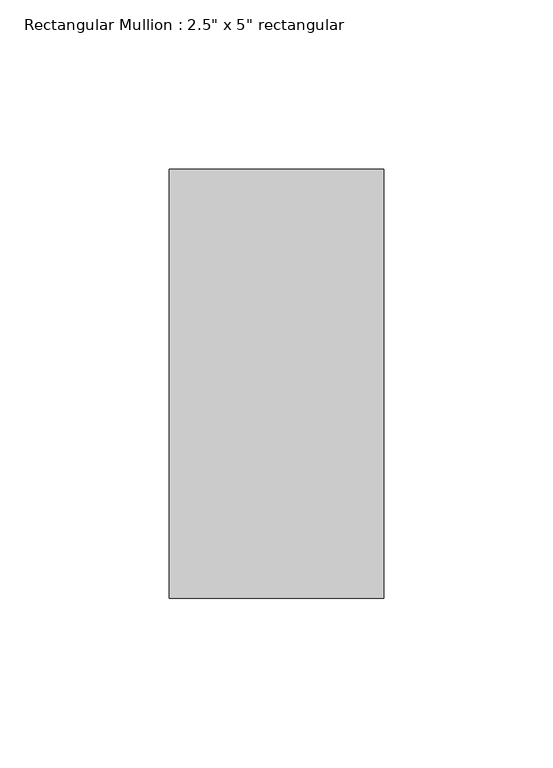
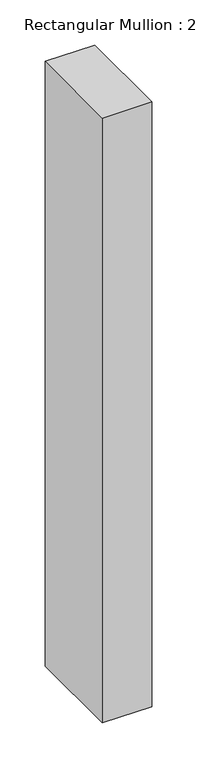
"""IFC4 building model written with IfcOpenShell, lengths in millimetres: member geometry."""

from ifc_helpers import new_model, si_unit, frame, origin, place, context, project, spatial, polyline, outline, extrude, source, transform, mapped, element, save


def member_ad567e07(model_context):
    return source(origin(), model_context, "Body", "SweptSolid", [
        extrude(outline(polyline([(31.75, 63.5), (31.75, -63.5), (-31.75, -63.5), (-31.75, 63.5), (31.75, 63.5)])), frame((0.0, 0.0, -819.15), z_axis=(0.0, 0.0, 1.0), x_axis=(1.0, 0.0, 0.0)), (0.0, 0.0, 1.0), 819.15),
    ])


if __name__ == "__main__":
    model = new_model("IFC4")
    model_context = context("Model", 3, world=origin())
    ifc_project = project(units=[si_unit("LENGTHUNIT", "METRE", prefix="MILLI")], contexts=[model_context])
    site = spatial("IfcSite", under=ifc_project)
    building = spatial("IfcBuilding", under=site)
    placement = place(None, origin())
    member_shape = member_ad567e07(model_context)
    element("IfcMember", 1, ObjectType="Rectangular Mullion : 2.5\" x 5\" rectangular", at=placement, inside=building, context=model_context, shape_type="MappedRepresentation", body=[
        mapped(member_shape, transform((0.0, 0.0, 0.0), x_axis=(1.0, 0.0, 0.0), y_axis=(0.0, 1.0, 0.0), z_axis=(0.0, 0.0, 1.0))),
    ])
    save(model, "model.ifc")

# Revit data of these elements
# Type "Rectangular Mullion : 2.5\" x 5\" rectangular"
#   built-in parameter 1007304 = 0.416667 (stored number, unit not read)
#   built-in parameter 1007301 = 0.104167 (stored number, unit not read)
#   built-in parameter 1007300 = 0.104167 (stored number, unit not read)
# Element 1 (IfcMember, "Rectangular Mullion : 2.5\" x 5\" rectangular")
#   Materials on its faces: "Aluminum"
# Materials
#   "Aluminum": class "Metal", colour RGB 247 247 247, transparency 0, Description = "Aluminum 6061", Cost = 0
